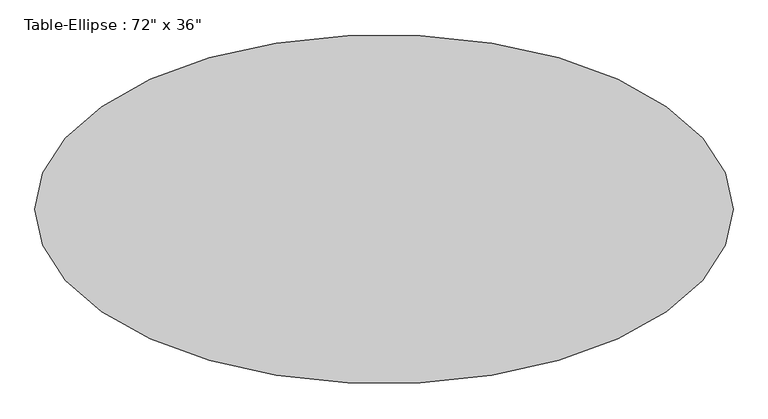
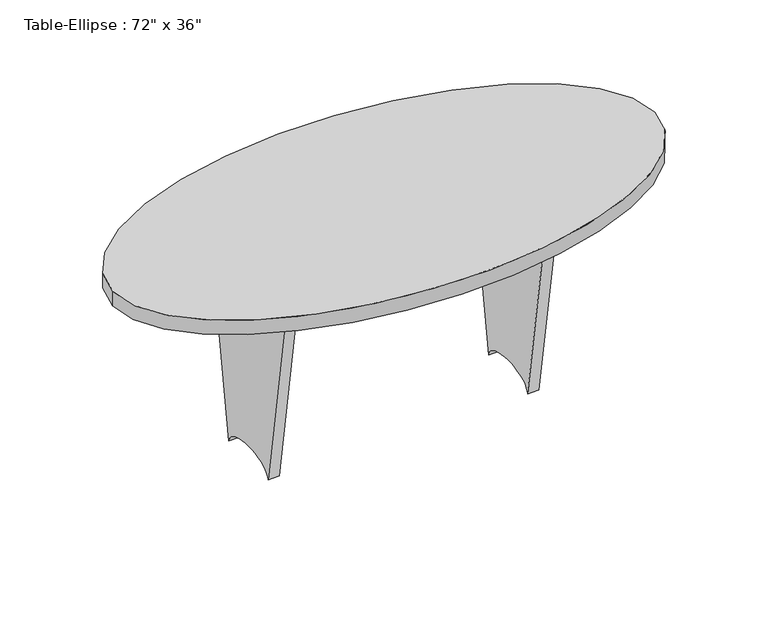
"""IFC4 building model written with IfcOpenShell, lengths in millimetres: furniture geometry."""

from ifc_helpers import new_model, si_unit, point, frame, origin, place, context, project, spatial, ellipse_curve, trimmed, source, transform, mapped, element, save
from ifc_brep_helpers import plane_surface, extruded_surface, advanced_brep


def furniture_15aefc23(model_context):
    return source(origin(), model_context, "Body", "AdvancedBrep", [
        advanced_brep(
        [(-914.4, 0.0, 762.0), (914.4, 0.0, 762.0), (-914.4, 0.0, 711.2), (914.4, 0.0, 711.2)],
        [
            (0, 1, ellipse_curve(frame((0.0, 0.0, 762.0), z_axis=(0.0, 0.0, 1.0), x_axis=(1.0, 0.0, 0.0)), 914.4, 457.2)),
            (1, 0, ellipse_curve(frame((0.0, 0.0, 762.0), z_axis=(0.0, 0.0, 1.0), x_axis=(1.0, 0.0, 0.0)), 914.4, 457.2)),
            (2, 3, ellipse_curve(frame((0.0, 0.0, 711.2), z_axis=(0.0, 0.0, -1.0), x_axis=(1.0, 0.0, 0.0)), 914.4, 457.2)),
            (3, 2, ellipse_curve(frame((0.0, 0.0, 711.2), z_axis=(0.0, 0.0, -1.0), x_axis=(1.0, 0.0, 0.0)), 914.4, 457.2)),
            (0, 2),
            (3, 1),
        ],
        [
            plane_surface(frame((914.4, 0.0, 762.0), z_axis=(0.0, 0.0, 1.0), x_axis=(0.0, 1.0, 0.0))),
            plane_surface(frame((914.4, 0.0, 711.2), z_axis=(0.0, 0.0, -1.0), x_axis=(0.0, -1.0, 0.0))),
            extruded_surface(trimmed(ellipse_curve(frame((0.0, 0.0, 660.4), z_axis=(0.0, 0.0, 1.0), x_axis=(1.0, 0.0, 0.0)), 914.4, 457.2), [point((-914.4, 0.0, 660.4))], [point((914.4, 0.0, 660.4))], True, "CARTESIAN"), (0.0, 0.0, 50.80000000000007), 50.80000000000007),
            extruded_surface(trimmed(ellipse_curve(frame((0.0, 0.0, 660.4), z_axis=(0.0, 0.0, 1.0), x_axis=(1.0, 0.0, 0.0)), 914.4, 457.2), [point((914.4, 0.0, 660.4))], [point((-914.4, 0.0, 660.4))], True, "CARTESIAN"), (0.0, 0.0, 50.80000000000007), 50.80000000000007),
        ],
        [
            (0, [[1, 2]]),
            (1, [[3, 4]]),
            (2, [[-1, 5, -4, 6]]),
            (3, [[-2, -6, -3, -5]]),
        ],
    ),
        advanced_brep(
        [(-419.1, 228.6, 711.2), (-419.1, -228.6, 711.2), (-419.1, -114.3, 0.0), (-419.1, 114.3, 0.0), (-457.2, 228.6, 711.2), (-457.2, 114.3, 0.0), (-457.2, -114.3, 0.0), (-457.2, -228.6, 711.2)],
        [
            (0, 1),
            (1, 2),
            (2, 3, ellipse_curve(frame((-419.1, 0.0, 0.0), z_axis=(-1.0, 0.0, 0.0), x_axis=(0.0, 1.0, 0.0)), 114.3, 50.8)),
            (3, 0),
            (4, 5),
            (5, 6, ellipse_curve(frame((-457.2, 0.0, 0.0), z_axis=(1.0, 0.0, 0.0), x_axis=(0.0, 1.0, 0.0)), 114.3, 50.8)),
            (6, 7),
            (7, 4),
            (0, 4),
            (7, 1),
            (6, 2),
            (5, 3),
        ],
        [
            plane_surface(frame((-419.1, -228.6, 711.2), z_axis=(1.0, 0.0, 0.0), x_axis=(0.0, -1.0, 0.0))),
            plane_surface(frame((-457.2, -228.6, 711.2), z_axis=(-1.0, 0.0, 0.0), x_axis=(0.0, 1.0, 0.0))),
            plane_surface(frame((-419.1, 228.6, 711.2), z_axis=(0.0, 0.0, 1.0), x_axis=(-1.0, 0.0, 0.0))),
            plane_surface(frame((-419.1, -228.6, 711.2), z_axis=(0.0, -0.9873303712766983, -0.15867809538375854), x_axis=(-1.0, 0.0, 0.0))),
            extruded_surface(trimmed(ellipse_curve(frame((-495.3, 0.0, 0.0), z_axis=(-1.0, 0.0, 0.0), x_axis=(0.0, 1.0, 0.0)), 114.3, 50.8), [point((-495.3, -114.3, 0.0))], [point((-495.3, 114.3, 0.0))], True, "CARTESIAN"), (38.10000000000002, 0.0, 0.0), 38.10000000000002),
            plane_surface(frame((-419.1, 114.3, 0.0), z_axis=(0.0, 0.9873303712766998, -0.15867809538374977), x_axis=(-1.0, 0.0, 0.0))),
        ],
        [
            (0, [[1, 2, 3, 4]]),
            (1, [[5, 6, 7, 8]]),
            (2, [[-1, 9, -8, 10]]),
            (3, [[-2, -10, -7, 11]]),
            (4, [[-3, -11, -6, 12]]),
            (5, [[-4, -12, -5, -9]]),
        ],
    ),
        advanced_brep(
        [(457.2, 228.6, 711.2), (457.2, -228.6, 711.2), (457.2, -114.3, 0.0), (457.2, 114.3, 0.0), (419.1, 228.6, 711.2), (419.1, 114.3, 0.0), (419.1, -114.3, 0.0), (419.1, -228.6, 711.2)],
        [
            (0, 1),
            (1, 2),
            (2, 3, ellipse_curve(frame((457.2, 0.0, 0.0), z_axis=(-1.0, 0.0, 0.0), x_axis=(0.0, 1.0, 0.0)), 114.3, 50.8)),
            (3, 0),
            (4, 5),
            (5, 6, ellipse_curve(frame((419.1, 0.0, 0.0), z_axis=(1.0, 0.0, 0.0), x_axis=(0.0, 1.0, 0.0)), 114.3, 50.8)),
            (6, 7),
            (7, 4),
            (0, 4),
            (7, 1),
            (6, 2),
            (5, 3),
        ],
        [
            plane_surface(frame((457.2, -228.6, 711.2), z_axis=(1.0, 0.0, 0.0), x_axis=(0.0, -1.0, 0.0))),
            plane_surface(frame((419.1, -228.6, 711.2), z_axis=(-1.0, 0.0, 0.0), x_axis=(0.0, 1.0, 0.0))),
            plane_surface(frame((457.2, 228.6, 711.2), z_axis=(0.0, 0.0, 1.0), x_axis=(-1.0, 0.0, 0.0))),
            plane_surface(frame((457.2, -228.6, 711.2), z_axis=(0.0, -0.9873303712766985, -0.15867809538375685), x_axis=(-1.0, 0.0, 0.0))),
            extruded_surface(trimmed(ellipse_curve(frame((381.0, 0.0, 0.0), z_axis=(-1.0, 0.0, 0.0), x_axis=(0.0, 1.0, 0.0)), 114.3, 50.8), [point((381.0, -114.3, 0.0))], [point((381.0, 114.3, 0.0))], True, "CARTESIAN"), (38.10000000000002, 0.0, 0.0), 38.10000000000002),
            plane_surface(frame((457.2, 114.3, 0.0), z_axis=(0.0, 0.9873303712767002, -0.15867809538374666), x_axis=(-1.0, 0.0, 0.0))),
        ],
        [
            (0, [[1, 2, 3, 4]]),
            (1, [[5, 6, 7, 8]]),
            (2, [[-1, 9, -8, 10]]),
            (3, [[-2, -10, -7, 11]]),
            (4, [[-3, -11, -6, 12]]),
            (5, [[-4, -12, -5, -9]]),
        ],
    ),
        advanced_brep(
        [(-419.1, 19.05, 711.2), (419.1, 19.05, 711.2), (419.1, 19.05, 474.1333333), (-419.1, 19.05, 474.1333333), (-419.1, -19.05, 711.2), (-419.1, -19.05, 474.1333333), (419.1, -19.05, 474.1333333), (419.1, -19.05, 711.2)],
        [
            (0, 1),
            (1, 2),
            (2, 3, ellipse_curve(frame((0.0, 19.05, 474.1333333), z_axis=(0.0, -1.0, 0.0), x_axis=(1.0, 0.0, 0.0)), 419.1, 101.6)),
            (3, 0),
            (4, 5),
            (5, 6, ellipse_curve(frame((0.0, -19.05, 474.1333333), z_axis=(0.0, 1.0, 0.0), x_axis=(1.0, 0.0, 0.0)), 419.1, 101.6)),
            (6, 7),
            (7, 4),
            (0, 4),
            (7, 1),
            (6, 2),
            (5, 3),
        ],
        [
            plane_surface(frame((-419.1, 19.05, 711.2), z_axis=(0.0, 1.0, 0.0), x_axis=(1.0, 0.0, 0.0))),
            plane_surface(frame((-419.1, -19.05, 711.2), z_axis=(0.0, -1.0, 0.0), x_axis=(-1.0, 0.0, 0.0))),
            plane_surface(frame((-419.1, 19.05, 711.2), z_axis=(0.0, 0.0, 1.0), x_axis=(0.0, -1.0, 0.0))),
            plane_surface(frame((419.1, 19.05, 711.2), z_axis=(1.0, 0.0, 0.0), x_axis=(0.0, -1.0, 0.0))),
            extruded_surface(trimmed(ellipse_curve(frame((0.0, -57.15, 474.1333333), z_axis=(0.0, -1.0, 0.0), x_axis=(1.0, 0.0, 0.0)), 419.1, 101.6), [point((419.1, -57.15, 474.1333333))], [point((-419.1, -57.15, 474.1333333))], True, "CARTESIAN"), (0.0, 38.099999999999994, 0.0), 38.099999999999994),
            plane_surface(frame((-419.1, 19.05, 474.1333333), z_axis=(-1.0, 0.0, 0.0), x_axis=(0.0, -1.0, 0.0))),
        ],
        [
            (0, [[1, 2, 3, 4]]),
            (1, [[5, 6, 7, 8]]),
            (2, [[-1, 9, -8, 10]]),
            (3, [[-2, -10, -7, 11]]),
            (4, [[-3, -11, -6, 12]]),
            (5, [[-4, -12, -5, -9]]),
        ],
    ),
    ])


if __name__ == "__main__":
    model = new_model("IFC4")
    model_context = context("Model", 3, world=origin())
    ifc_project = project(units=[si_unit("LENGTHUNIT", "METRE", prefix="MILLI")], contexts=[model_context])
    site = spatial("IfcSite", under=ifc_project)
    building = spatial("IfcBuilding", under=site)
    placement = place(None, origin())
    furniture_shape = furniture_15aefc23(model_context)
    element("IfcFurniture", 1, ObjectType="Table-Ellipse : 72\" x 36\"", at=placement, inside=building, context=model_context, shape_type="MappedRepresentation", body=[
        mapped(furniture_shape, transform((0.0, 0.0, 0.0), x_axis=(1.0, 0.0, 0.0), y_axis=(0.0, 1.0, 0.0), z_axis=(0.0, 0.0, 1.0))),
    ])
    save(model, "model.ifc")

# Revit data of these elements
# Type "Table-Ellipse : 72\" x 36\""
#   Assembly Code = "E2020200"
#   Half Width = 1' - 6"
#   Half Length = 3' - 0"
#   Height = 2' - 6"
#   Length = 6' - 0"
#   Width = 3' - 0"
#   Base Material = Birch
#   Top Material = Laminate - Black
#   Default Elevation = 0
# Element 1 (IfcFurniture, "Table-Ellipse : 72\" x 36\"")
#   Materials on its faces: "Birch", "Laminate - Black"
# Materials
#   "Birch": class "Wood", colour RGB 224 178 126, transparency 0, Description = "Betula Alleghaniensis", Cost = 0
#   "Laminate - Black": colour RGB 0 0 0, transparency 0
